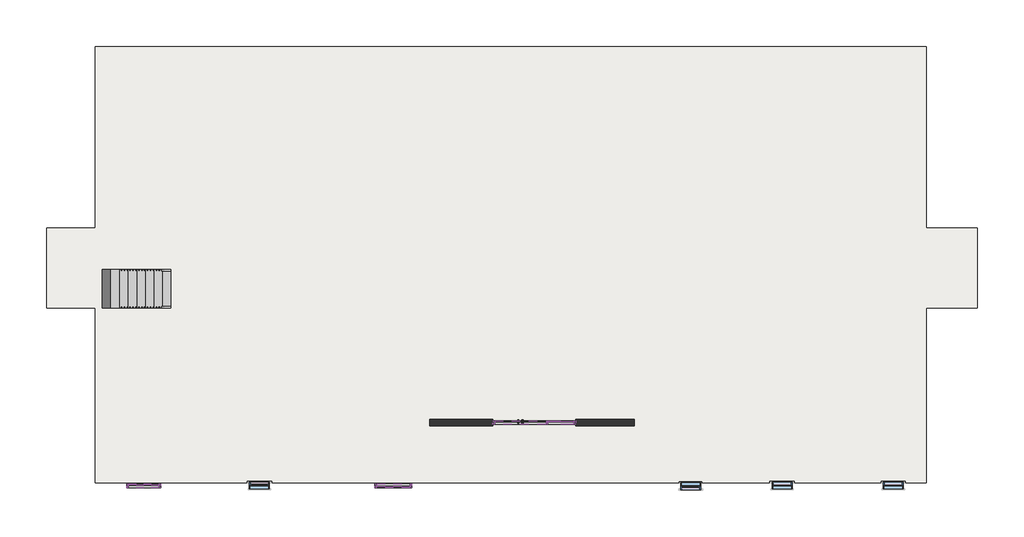
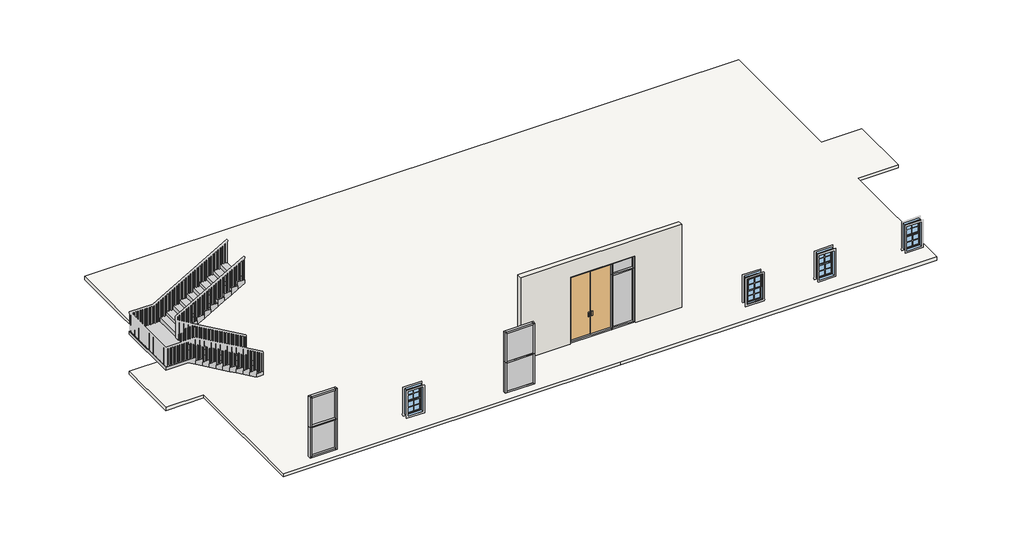
# One storey, part 1 of 3: 25 members, 6 plates, 4 windows, 1 door, 1 slab, 1 stair flight, 1 wall.
"""IFC4 building model written with IfcOpenShell, lengths in millimetres."""

from ifc_helpers import new_model, si_unit, frame, origin, place, context, project, spatial, polyline, outline, extrude, faceted_brep, transform, mapped, element, save
from components import m_door_curtain_wall_double_glass_m_door_curtain_wall_double_f99ce068, rectangular_mullion_65_x_125mm_rectangular_b7ff14d5, rectangular_mullion_65_x_125mm_rectangular_013ac084, rectangular_mullion_65_x_125mm_rectangular_ca84e85e, rectangular_mullion_65_x_125mm_rectangular_f4cebacc, rectangular_mullion_65_x_125mm_rectangular_d33d7bb0, rectangular_mullion_65_x_125mm_rectangular_fcec82ed, rectangular_mullion_65_x_125mm_rectangular_cb623ca7, rectangular_mullion_65_x_125mm_rectangular_e22a5c8f, rectangular_mullion_65_x_125mm_rectangular_b6b0b808, rectangular_mullion_65_x_125mm_rectangular_89386302, rectangular_mullion_65_x_125mm_rectangular_1b222a86, rectangular_mullion_65_x_125mm_rectangular_018360c9, system_panel_glazed_abc17199, system_panel_glazed_3f3a89de, system_panel_glazed_39fbb70d, system_panel_glazed_1607d5b8, m_window_double_hung_700_x_1200mm_9cb858e8

model = new_model("IFC4")

# Units and contexts
model_context = context("Model", 3, world=origin())
ifc_project = project(units=[si_unit("LENGTHUNIT", "METRE", prefix="MILLI")], contexts=[model_context])

# Site, building, storey
site = spatial("IfcSite", under=ifc_project)
building = spatial("IfcBuilding", under=site)
storey = spatial("IfcBuildingStorey", under=building, Elevation=600.0)

# Door
placement = place(None, origin())
m_door_curtain_wall_double_glass_m_door_curtain_wall_double_shape = m_door_curtain_wall_double_glass_m_door_curtain_wall_double_f99ce068(model_context)
element("IfcDoor", 1, ObjectType="M_Door-Curtain-Wall-Double-Glass : M_Door-Curtain-Wall-Double-Glass", at=placement, inside=storey, context=model_context, shape_type="MappedRepresentation", body=[
    mapped(m_door_curtain_wall_double_glass_m_door_curtain_wall_double_shape, transform((5384.8330368, -10653.0592374, 665.0), x_axis=(1.0, 0.0, 0.0), y_axis=(0.0, 1.0, 0.0), z_axis=(0.0, 0.0, 1.0))),
])

# Members
rectangular_mullion_65_x_125mm_rectangular_shape = rectangular_mullion_65_x_125mm_rectangular_b7ff14d5(model_context)
element("IfcMember", 2, ObjectType="Rectangular Mullion : 65 x 125mm rectangular", at=placement, inside=storey, context=model_context, shape_type="MappedRepresentation", body=[
    mapped(rectangular_mullion_65_x_125mm_rectangular_shape, transform((-7258.9169632, -12865.5592374, 3900.0), x_axis=(0.0, 0.0, 1.0), y_axis=(0.0, -1.0, 0.0), z_axis=(1.0, 0.0, 0.0))),
])
element("IfcMember", 3, ObjectType="Rectangular Mullion : 65 x 125mm rectangular", at=placement, inside=storey, context=model_context, shape_type="MappedRepresentation", body=[
    mapped(rectangular_mullion_65_x_125mm_rectangular_shape, transform((-8328.9169632, -12865.5592374, 1050.0), x_axis=(0.0, 0.0, -1.0), y_axis=(0.0, -1.0, 0.0), z_axis=(-1.0, 0.0, 0.0))),
])
rectangular_mullion_65_x_125mm_rectangular_2_shape = rectangular_mullion_65_x_125mm_rectangular_013ac084(model_context)
element("IfcMember", 4, ObjectType="Rectangular Mullion : 65 x 125mm rectangular", at=placement, inside=storey, context=model_context, shape_type="MappedRepresentation", body=[
    mapped(rectangular_mullion_65_x_125mm_rectangular_2_shape, transform((358.5830368, -12865.5592374, 3900.0), x_axis=(0.0, 0.0, 1.0), y_axis=(0.0, 1.0, 0.0), z_axis=(-1.0, 0.0, 0.0))),
])
element("IfcMember", 5, ObjectType="Rectangular Mullion : 65 x 125mm rectangular", at=placement, inside=storey, context=model_context, shape_type="MappedRepresentation", body=[
    mapped(rectangular_mullion_65_x_125mm_rectangular_2_shape, transform((1528.5830368, -12865.5592374, 1050.0), x_axis=(0.0, 0.0, -1.0), y_axis=(0.0, 1.0, 0.0), z_axis=(1.0, 0.0, 0.0))),
])
rectangular_mullion_65_x_125mm_rectangular_3_shape = rectangular_mullion_65_x_125mm_rectangular_ca84e85e(model_context)
element("IfcMember", 6, ObjectType="Rectangular Mullion : 65 x 125mm rectangular", at=placement, inside=storey, context=model_context, shape_type="MappedRepresentation", body=[
    mapped(rectangular_mullion_65_x_125mm_rectangular_3_shape, transform((-7258.9169632, -12865.5592374, 2475.0), x_axis=(0.0, 0.0, 1.0), y_axis=(0.0, -1.0, 0.0), z_axis=(1.0, 0.0, 0.0))),
])
rectangular_mullion_65_x_125mm_rectangular_4_shape = rectangular_mullion_65_x_125mm_rectangular_f4cebacc(model_context)
element("IfcMember", 7, ObjectType="Rectangular Mullion : 65 x 125mm rectangular", at=placement, inside=storey, context=model_context, shape_type="MappedRepresentation", body=[
    mapped(rectangular_mullion_65_x_125mm_rectangular_4_shape, transform((-7193.9169632, -12865.5592374, 1050.0), x_axis=(1.0, 0.0, 0.0), y_axis=(0.0, -1.0, 0.0), z_axis=(0.0, 0.0, -1.0))),
])
element("IfcMember", 8, ObjectType="Rectangular Mullion : 65 x 125mm rectangular", at=placement, inside=storey, context=model_context, shape_type="MappedRepresentation", body=[
    mapped(rectangular_mullion_65_x_125mm_rectangular_4_shape, transform((293.5830368, -12865.5592374, 1050.0), x_axis=(-1.0, 0.0, 0.0), y_axis=(0.0, 1.0, 0.0), z_axis=(0.0, 0.0, -1.0))),
])
element("IfcMember", 9, ObjectType="Rectangular Mullion : 65 x 125mm rectangular", at=placement, inside=storey, context=model_context, shape_type="MappedRepresentation", body=[
    mapped(rectangular_mullion_65_x_125mm_rectangular_4_shape, transform((-8393.9169632, -12865.5592374, 3900.0), x_axis=(-1.0, 0.0, 0.0), y_axis=(0.0, -1.0, 0.0), z_axis=(0.0, 0.0, 1.0))),
])
element("IfcMember", 10, ObjectType="Rectangular Mullion : 65 x 125mm rectangular", at=placement, inside=storey, context=model_context, shape_type="MappedRepresentation", body=[
    mapped(rectangular_mullion_65_x_125mm_rectangular_4_shape, transform((1593.5830368, -12865.5592374, 3900.0), x_axis=(1.0, 0.0, 0.0), y_axis=(0.0, 1.0, 0.0), z_axis=(0.0, 0.0, 1.0))),
])
element("IfcMember", 11, ObjectType="Rectangular Mullion : 65 x 125mm rectangular", at=placement, inside=storey, context=model_context, shape_type="MappedRepresentation", body=[
    mapped(rectangular_mullion_65_x_125mm_rectangular_4_shape, transform((293.5830368, -12865.5592374, 2475.0), x_axis=(-1.0, 0.0, 0.0), y_axis=(0.0, 1.0, 0.0), z_axis=(0.0, 0.0, -1.0))),
])
element("IfcMember", 12, ObjectType="Rectangular Mullion : 65 x 125mm rectangular", at=placement, inside=storey, context=model_context, shape_type="MappedRepresentation", body=[
    mapped(rectangular_mullion_65_x_125mm_rectangular_4_shape, transform((-7193.9169632, -12865.5592374, 2475.0), x_axis=(1.0, 0.0, 0.0), y_axis=(0.0, -1.0, 0.0), z_axis=(0.0, 0.0, -1.0))),
])
element("IfcMember", 13, ObjectType="Rectangular Mullion : 65 x 125mm rectangular", at=placement, inside=storey, context=model_context, shape_type="MappedRepresentation", body=[
    mapped(rectangular_mullion_65_x_125mm_rectangular_4_shape, transform((1593.5830368, -12865.5592374, 2475.0), x_axis=(1.0, 0.0, 0.0), y_axis=(0.0, 1.0, 0.0), z_axis=(0.0, 0.0, 1.0))),
])
element("IfcMember", 14, ObjectType="Rectangular Mullion : 65 x 125mm rectangular", at=placement, inside=storey, context=model_context, shape_type="MappedRepresentation", body=[
    mapped(rectangular_mullion_65_x_125mm_rectangular_4_shape, transform((-8393.9169632, -12865.5592374, 2475.0), x_axis=(-1.0, 0.0, 0.0), y_axis=(0.0, -1.0, 0.0), z_axis=(0.0, 0.0, 1.0))),
])
rectangular_mullion_65_x_125mm_rectangular_5_shape = rectangular_mullion_65_x_125mm_rectangular_d33d7bb0(model_context)
element("IfcMember", 15, ObjectType="Rectangular Mullion : 65 x 125mm rectangular", at=placement, inside=storey, context=model_context, shape_type="MappedRepresentation", body=[
    mapped(rectangular_mullion_65_x_125mm_rectangular_5_shape, transform((358.5830368, -12865.5592374, 2475.0), x_axis=(0.0, 0.0, 1.0), y_axis=(0.0, 1.0, 0.0), z_axis=(-1.0, 0.0, 0.0))),
])
rectangular_mullion_65_x_125mm_rectangular_6_shape = rectangular_mullion_65_x_125mm_rectangular_fcec82ed(model_context)
element("IfcMember", 16, ObjectType="Rectangular Mullion : 65 x 125mm rectangular", at=placement, inside=storey, context=model_context, shape_type="MappedRepresentation", body=[
    mapped(rectangular_mullion_65_x_125mm_rectangular_6_shape, transform((7253.5830368, -10653.0592374, 3750.0), x_axis=(0.0, 0.0, 1.0), y_axis=(0.0, -1.0, 0.0), z_axis=(1.0, 0.0, 0.0))),
])
rectangular_mullion_65_x_125mm_rectangular_7_shape = rectangular_mullion_65_x_125mm_rectangular_cb623ca7(model_context)
element("IfcMember", 17, ObjectType="Rectangular Mullion : 65 x 125mm rectangular", at=placement, inside=storey, context=model_context, shape_type="MappedRepresentation", body=[
    mapped(rectangular_mullion_65_x_125mm_rectangular_7_shape, transform((4483.5830368, -10653.0592374, 600.0), x_axis=(0.0, 0.0, -1.0), y_axis=(0.0, -1.0, 0.0), z_axis=(-1.0, 0.0, 0.0))),
])
element("IfcMember", 18, ObjectType="Rectangular Mullion : 65 x 125mm rectangular", at=placement, inside=storey, context=model_context, shape_type="MappedRepresentation", body=[
    mapped(rectangular_mullion_65_x_125mm_rectangular_7_shape, transform((6286.0830368, -10653.0592374, 3750.0), x_axis=(0.0, 0.0, 1.0), y_axis=(0.0, -1.0, 0.0), z_axis=(1.0, 0.0, 0.0))),
])
element("IfcMember", 19, ObjectType="Rectangular Mullion : 65 x 125mm rectangular", at=placement, inside=storey, context=model_context, shape_type="MappedRepresentation", body=[
    mapped(rectangular_mullion_65_x_125mm_rectangular_6_shape, transform((6351.0830368, -10653.0592374, 600.0), x_axis=(0.0, 0.0, -1.0), y_axis=(0.0, -1.0, 0.0), z_axis=(-1.0, 0.0, 0.0))),
])
rectangular_mullion_65_x_125mm_rectangular_8_shape = rectangular_mullion_65_x_125mm_rectangular_e22a5c8f(model_context)
element("IfcMember", 20, ObjectType="Rectangular Mullion : 65 x 125mm rectangular", at=placement, inside=storey, context=model_context, shape_type="MappedRepresentation", body=[
    mapped(rectangular_mullion_65_x_125mm_rectangular_8_shape, transform((4418.5830368, -10653.0592374, 3750.0), x_axis=(-1.0, 0.0, 0.0), y_axis=(0.0, -1.0, 0.0), z_axis=(0.0, 0.0, 1.0))),
])
rectangular_mullion_65_x_125mm_rectangular_9_shape = rectangular_mullion_65_x_125mm_rectangular_b6b0b808(model_context)
element("IfcMember", 21, ObjectType="Rectangular Mullion : 65 x 125mm rectangular", at=placement, inside=storey, context=model_context, shape_type="MappedRepresentation", body=[
    mapped(rectangular_mullion_65_x_125mm_rectangular_9_shape, transform((4418.5830368, -10653.0592374, 3150.0), x_axis=(-1.0, 0.0, 0.0), y_axis=(0.0, -1.0, 0.0), z_axis=(0.0, 0.0, 1.0))),
])
rectangular_mullion_65_x_125mm_rectangular_10_shape = rectangular_mullion_65_x_125mm_rectangular_89386302(model_context)
element("IfcMember", 22, ObjectType="Rectangular Mullion : 65 x 125mm rectangular", at=placement, inside=storey, context=model_context, shape_type="MappedRepresentation", body=[
    mapped(rectangular_mullion_65_x_125mm_rectangular_10_shape, transform((6318.5830368, -10653.0592374, 600.0), x_axis=(1.0, 0.0, 0.0), y_axis=(0.0, -1.0, 0.0), z_axis=(0.0, 0.0, -1.0))),
])
rectangular_mullion_65_x_125mm_rectangular_11_shape = rectangular_mullion_65_x_125mm_rectangular_1b222a86(model_context)
element("IfcMember", 23, ObjectType="Rectangular Mullion : 65 x 125mm rectangular", at=placement, inside=storey, context=model_context, shape_type="MappedRepresentation", body=[
    mapped(rectangular_mullion_65_x_125mm_rectangular_11_shape, transform((6318.5830368, -10653.0592374, 3150.0), x_axis=(1.0, 0.0, 0.0), y_axis=(0.0, -1.0, 0.0), z_axis=(0.0, 0.0, -1.0))),
])
rectangular_mullion_65_x_125mm_rectangular_12_shape = rectangular_mullion_65_x_125mm_rectangular_018360c9(model_context)
element("IfcMember", 24, ObjectType="Rectangular Mullion : 65 x 125mm rectangular", at=placement, inside=storey, context=model_context, shape_type="MappedRepresentation", body=[
    mapped(rectangular_mullion_65_x_125mm_rectangular_12_shape, transform((7253.5830368, -10653.0592374, 3150.0), x_axis=(0.0, 0.0, 1.0), y_axis=(0.0, -1.0, 0.0), z_axis=(1.0, 0.0, 0.0))),
])
element("IfcMember", 25, ObjectType="Rectangular Mullion : 65 x 125mm rectangular", at=placement, inside=storey, context=model_context, shape_type="MappedRepresentation", body=[
    mapped(rectangular_mullion_65_x_125mm_rectangular_9_shape, transform((7318.5830368, -10653.0592374, 600.0), x_axis=(1.0, 0.0, 0.0), y_axis=(0.0, -1.0, 0.0), z_axis=(0.0, 0.0, -1.0))),
])
element("IfcMember", 26, ObjectType="Rectangular Mullion : 65 x 125mm rectangular", at=placement, inside=storey, context=model_context, shape_type="MappedRepresentation", body=[
    mapped(rectangular_mullion_65_x_125mm_rectangular_8_shape, transform((7318.5830368, -10653.0592374, 3150.0), x_axis=(1.0, 0.0, 0.0), y_axis=(0.0, -1.0, 0.0), z_axis=(0.0, 0.0, -1.0))),
])

# Plates
system_panel_glazed_shape = system_panel_glazed_abc17199(model_context)
element("IfcPlate", 27, ObjectType="System Panel : Glazed", at=placement, inside=storey, context=model_context, shape_type="MappedRepresentation", body=[
    mapped(system_panel_glazed_shape, transform((-7793.9169632, -12865.5592374, 1115.0), x_axis=(1.0, 0.0, 0.0), y_axis=(0.0, 1.0, 0.0), z_axis=(0.0, 0.0, 1.0))),
])
element("IfcPlate", 28, ObjectType="System Panel : Glazed", at=placement, inside=storey, context=model_context, shape_type="MappedRepresentation", body=[
    mapped(system_panel_glazed_shape, transform((-7793.9169632, -12865.5592374, 2507.5), x_axis=(1.0, 0.0, 0.0), y_axis=(0.0, 1.0, 0.0), z_axis=(0.0, 0.0, 1.0))),
])
system_panel_glazed_2_shape = system_panel_glazed_3f3a89de(model_context)
element("IfcPlate", 29, ObjectType="System Panel : Glazed", at=placement, inside=storey, context=model_context, shape_type="MappedRepresentation", body=[
    mapped(system_panel_glazed_2_shape, transform((943.5830368, -12865.5592374, 1115.0), x_axis=(-1.0, 0.0, 0.0), y_axis=(0.0, -1.0, 0.0), z_axis=(0.0, 0.0, 1.0))),
])
element("IfcPlate", 30, ObjectType="System Panel : Glazed", at=placement, inside=storey, context=model_context, shape_type="MappedRepresentation", body=[
    mapped(system_panel_glazed_2_shape, transform((943.5830368, -12865.5592374, 2507.5), x_axis=(-1.0, 0.0, 0.0), y_axis=(0.0, -1.0, 0.0), z_axis=(0.0, 0.0, 1.0))),
])
system_panel_glazed_3_shape = system_panel_glazed_39fbb70d(model_context)
element("IfcPlate", 31, ObjectType="System Panel : Glazed", at=placement, inside=storey, context=model_context, shape_type="MappedRepresentation", body=[
    mapped(system_panel_glazed_3_shape, transform((6802.3330368, -10653.0592374, 665.0), x_axis=(1.0, 0.0, 0.0), y_axis=(0.0, 1.0, 0.0), z_axis=(0.0, 0.0, 1.0))),
])
system_panel_glazed_4_shape = system_panel_glazed_1607d5b8(model_context)
element("IfcPlate", 32, ObjectType="System Panel : Glazed", at=placement, inside=storey, context=model_context, shape_type="MappedRepresentation", body=[
    mapped(system_panel_glazed_4_shape, transform((6802.3330368, -10653.0592374, 3182.5), x_axis=(1.0, 0.0, 0.0), y_axis=(0.0, 1.0, 0.0), z_axis=(0.0, 0.0, 1.0))),
])

# Slab
element("IfcSlab", 33, ObjectType="01-150 floor", at=placement, inside=storey, context=model_context, shape_type="SweptSolid", body=[
    extrude(outline(polyline([(-9493.9169632, 2521.9407626), (19581.0830368, 2521.9407626), (19581.0830368, -3840.5592374), (21381.0830368, -3840.5592374), (21381.0830368, -6640.5592374), (19581.0830368, -6640.5592374), (19581.0830368, -12753.0592374), (5529.3260748, -12753.0592374), (-9493.9169632, -12753.0592374), (-9493.9169632, -6640.5592374), (-11193.9169632, -6640.5592374), (-11193.9169632, -3840.5592374), (-9493.9169632, -3840.5592374), (-9493.9169632, 2521.9407626)])), frame((0.0, 0.0, 450.0), z_axis=(0.0, 0.0, 1.0), x_axis=(1.0, 0.0, 0.0)), (0.0, 0.0, 1.0), 150.0),
])

# Stair flight
element("IfcStairFlight", 34, ObjectType="M_Monolithic Run", at=placement, inside=storey, context=model_context, shape_type="Brep", body=[
    faceted_brep([(-7143.9169632, -6640.5592374, 771.4285714), (-6843.9169632, -6640.5592374, 771.4285714), (-6843.9169632, -5290.5592374, 771.4285714), (-7143.9169632, -5290.5592374, 771.4285714), (-7143.9169632, -6640.5592374, 600.0), (-6843.9169632, -6640.5592374, 600.0), (-6843.9169632, -5290.5592374, 600.0), (-7143.9169632, -5290.5592374, 600.0), (-7443.9169632, -6640.5592374, 942.8571429), (-7143.9169632, -6640.5592374, 942.8571429), (-7143.9169632, -5290.5592374, 942.8571429), (-7443.9169632, -5290.5592374, 942.8571429), (-7443.9169632, -6640.5592374, 770.0944768), (-7146.2516288, -6640.5592374, 600.0), (-7146.2516288, -5290.5592374, 600.0), (-7443.9169632, -5290.5592374, 770.0944768), (-7743.9169632, -6640.5592374, 1114.2857143), (-7443.9169632, -6640.5592374, 1114.2857143), (-7443.9169632, -5290.5592374, 1114.2857143), (-7743.9169632, -5290.5592374, 1114.2857143), (-7743.9169632, -6640.5592374, 941.5230483), (-7743.9169632, -5290.5592374, 941.5230483), (-8043.9169632, -6640.5592374, 1285.7142857), (-7743.9169632, -6640.5592374, 1285.7142857), (-7743.9169632, -5290.5592374, 1285.7142857), (-8043.9169632, -5290.5592374, 1285.7142857), (-8043.9169632, -6640.5592374, 1112.9516197), (-8043.9169632, -5290.5592374, 1112.9516197), (-8343.9169632, -6640.5592374, 1457.1428571), (-8043.9169632, -6640.5592374, 1457.1428571), (-8043.9169632, -5290.5592374, 1457.1428571), (-8343.9169632, -5290.5592374, 1457.1428571), (-8343.9169632, -6640.5592374, 1284.3801911), (-8343.9169632, -5290.5592374, 1284.3801911), (-8643.9169632, -6640.5592374, 1628.5714286), (-8343.9169632, -6640.5592374, 1628.5714286), (-8343.9169632, -5290.5592374, 1628.5714286), (-8643.9169632, -5290.5592374, 1628.5714286), (-8643.9169632, -6640.5592374, 1455.8087625), (-8643.9169632, -5290.5592374, 1455.8087625), (-8943.9169632, -6640.5592374, 1800.0), (-8643.9169632, -6640.5592374, 1800.0), (-8643.9169632, -5290.5592374, 1800.0), (-8943.9169632, -5290.5592374, 1800.0), (-8943.9169632, -6640.5592374, 1627.237334), (-8943.9169632, -5290.5592374, 1627.237334), (-9243.9169632, -6640.5592374, 1971.4285714), (-8943.9169632, -6640.5592374, 1971.4285714), (-8943.9169632, -5290.5592374, 1971.4285714), (-9243.9169632, -5290.5592374, 1971.4285714), (-9243.9169632, -6640.5592374, 1798.6659054), (-9243.9169632, -5290.5592374, 1798.6659054), (-9543.9169632, -6640.5592374, 2142.8571429), (-9243.9169632, -6640.5592374, 2142.8571429), (-9243.9169632, -5290.5592374, 2142.8571429), (-9543.9169632, -5290.5592374, 2142.8571429), (-9543.9169632, -6640.5592374, 1970.0944768), (-9543.9169632, -5290.5592374, 1970.0944768), (-9843.9169632, -6640.5592374, 2314.2857143), (-9543.9169632, -6640.5592374, 2314.2857143), (-9543.9169632, -5290.5592374, 2314.2857143), (-9843.9169632, -5290.5592374, 2314.2857143), (-9843.9169632, -6640.5592374, 2141.5230483), (-10183.7516288, -5290.5592374, 2335.7142857), (-9843.9169632, -5290.5592374, 2335.7142857), (-9843.9169632, -3840.5592374, 2485.7142857), (-11193.9169632, -3840.5592374, 2485.7142857), (-11193.9169632, -6640.5592374, 2485.7142857), (-10183.7516288, -6640.5592374, 2485.7142857), (-9843.9169632, -6640.5592374, 2485.7142857), (-9843.9169632, -5290.5592374, 2485.7142857), (-9843.9169632, -5190.5592374, 2485.7142857), (-9843.9169632, -3840.5592374, 2335.7142857), (-11193.9169632, -3840.5592374, 2335.7142857), (-11193.9169632, -6640.5592374, 2335.7142857), (-10183.7516288, -6640.5592374, 2335.7142857), (-9843.9169632, -5190.5592374, 2335.7142857), (-9843.9169632, -3840.5592374, 2657.1428571), (-9843.9169632, -5190.5592374, 2657.1428571), (-9804.0822977, -5190.5592374, 2657.1428571), (-9543.9169632, -5190.5592374, 2657.1428571), (-9543.9169632, -3840.5592374, 2657.1428571), (-9804.0822977, -3840.5592374, 2657.1428571), (-9543.9169632, -3840.5592374, 2484.3801911), (-9804.0822977, -3840.5592374, 2335.7142857), (-9804.0822977, -5190.5592374, 2335.7142857), (-9543.9169632, -5190.5592374, 2484.3801911), (-9243.9169632, -3840.5592374, 2828.5714286), (-9543.9169632, -3840.5592374, 2828.5714286), (-9543.9169632, -5190.5592374, 2828.5714286), (-9243.9169632, -5190.5592374, 2828.5714286), (-9243.9169632, -3840.5592374, 2655.8087625), (-9243.9169632, -5190.5592374, 2655.8087625), (-8943.9169632, -3840.5592374, 3000.0), (-9243.9169632, -3840.5592374, 3000.0), (-9243.9169632, -5190.5592374, 3000.0), (-8943.9169632, -5190.5592374, 3000.0), (-8943.9169632, -3840.5592374, 2827.237334), (-8943.9169632, -5190.5592374, 2827.237334), (-8643.9169632, -3840.5592374, 3171.4285714), (-8943.9169632, -3840.5592374, 3171.4285714), (-8943.9169632, -5190.5592374, 3171.4285714), (-8643.9169632, -5190.5592374, 3171.4285714), (-8643.9169632, -3840.5592374, 2998.6659054), (-8643.9169632, -5190.5592374, 2998.6659054), (-8343.9169632, -3840.5592374, 3342.8571429), (-8643.9169632, -3840.5592374, 3342.8571429), (-8643.9169632, -5190.5592374, 3342.8571429), (-8343.9169632, -5190.5592374, 3342.8571429), (-8343.9169632, -3840.5592374, 3170.0944768), (-8343.9169632, -5190.5592374, 3170.0944768), (-8043.9169632, -3840.5592374, 3514.2857143), (-8343.9169632, -3840.5592374, 3514.2857143), (-8343.9169632, -5190.5592374, 3514.2857143), (-8043.9169632, -5190.5592374, 3514.2857143), (-8043.9169632, -3840.5592374, 3341.5230483), (-8043.9169632, -5190.5592374, 3341.5230483), (-7743.9169632, -3840.5592374, 3685.7142857), (-8043.9169632, -3840.5592374, 3685.7142857), (-8043.9169632, -5190.5592374, 3685.7142857), (-7743.9169632, -5190.5592374, 3685.7142857), (-7743.9169632, -3840.5592374, 3512.9516197), (-7743.9169632, -5190.5592374, 3512.9516197), (-7443.9169632, -3840.5592374, 3857.1428571), (-7743.9169632, -3840.5592374, 3857.1428571), (-7743.9169632, -5190.5592374, 3857.1428571), (-7443.9169632, -5190.5592374, 3857.1428571), (-7443.9169632, -3840.5592374, 3684.3801911), (-7443.9169632, -5190.5592374, 3684.3801911), (-7143.9169632, -3840.5592374, 4028.5714286), (-7443.9169632, -3840.5592374, 4028.5714286), (-7443.9169632, -5190.5592374, 4028.5714286), (-7143.9169632, -5190.5592374, 4028.5714286), (-7143.9169632, -3840.5592374, 3855.8087625), (-7143.9169632, -5190.5592374, 3855.8087625), (-6843.9169632, -3840.5592374, 4200.0), (-7143.9169632, -3840.5592374, 4200.0), (-7143.9169632, -5190.5592374, 4200.0), (-6843.9169632, -5190.5592374, 4200.0), (-6843.9169632, -3840.5592374, 4027.237334), (-6843.9169632, -5190.5592374, 4027.237334)], [[[0, 1, 2, 3]], [[1, 0, 4, 5]], [[2, 1, 5, 6]], [[3, 2, 6, 7]], [[8, 9, 10, 11]], [[4, 0, 9, 8, 12, 13]], [[0, 3, 10, 9]], [[3, 7, 14, 15, 11, 10]], [[16, 17, 18, 19]], [[17, 16, 20, 12, 8]], [[8, 11, 18, 17]], [[19, 18, 11, 15, 21]], [[22, 23, 24, 25]], [[23, 22, 26, 20, 16]], [[16, 19, 24, 23]], [[25, 24, 19, 21, 27]], [[28, 29, 30, 31]], [[29, 28, 32, 26, 22]], [[22, 25, 30, 29]], [[31, 30, 25, 27, 33]], [[34, 35, 36, 37]], [[35, 34, 38, 32, 28]], [[28, 31, 36, 35]], [[37, 36, 31, 33, 39]], [[40, 41, 42, 43]], [[41, 40, 44, 38, 34]], [[34, 37, 42, 41]], [[43, 42, 37, 39, 45]], [[46, 47, 48, 49]], [[47, 46, 50, 44, 40]], [[40, 43, 48, 47]], [[49, 48, 43, 45, 51]], [[52, 53, 54, 55]], [[53, 52, 56, 50, 46]], [[46, 49, 54, 53]], [[55, 54, 49, 51, 57]], [[58, 59, 60, 61]], [[59, 58, 62, 56, 52]], [[52, 55, 60, 59]], [[61, 60, 55, 57, 63, 64]], [[65, 66, 67, 68, 69, 70, 71]], [[66, 65, 72, 73]], [[67, 66, 73, 74]], [[58, 69, 68, 67, 74, 75, 62]], [[58, 61, 64, 70, 69]], [[71, 70, 64, 76]], [[77, 78, 79, 80, 81, 82]], [[65, 77, 82, 81, 83, 84, 72]], [[65, 71, 78, 77]], [[78, 71, 76, 85, 86, 80, 79]], [[87, 88, 89, 90]], [[88, 87, 91, 83, 81]], [[81, 80, 89, 88]], [[90, 89, 80, 86, 92]], [[93, 94, 95, 96]], [[94, 93, 97, 91, 87]], [[87, 90, 95, 94]], [[96, 95, 90, 92, 98]], [[99, 100, 101, 102]], [[100, 99, 103, 97, 93]], [[93, 96, 101, 100]], [[102, 101, 96, 98, 104]], [[105, 106, 107, 108]], [[106, 105, 109, 103, 99]], [[99, 102, 107, 106]], [[108, 107, 102, 104, 110]], [[111, 112, 113, 114]], [[112, 111, 115, 109, 105]], [[105, 108, 113, 112]], [[114, 113, 108, 110, 116]], [[117, 118, 119, 120]], [[118, 117, 121, 115, 111]], [[111, 114, 119, 118]], [[120, 119, 114, 116, 122]], [[123, 124, 125, 126]], [[124, 123, 127, 121, 117]], [[117, 120, 125, 124]], [[126, 125, 120, 122, 128]], [[129, 130, 131, 132]], [[130, 129, 133, 127, 123]], [[123, 126, 131, 130]], [[132, 131, 126, 128, 134]], [[135, 136, 137, 138]], [[136, 135, 139, 133, 129]], [[129, 132, 137, 136]], [[138, 137, 132, 134, 140]], [[135, 138, 140, 139]], [[5, 4, 13, 14, 7, 6]], [[75, 63, 57, 51, 45, 39, 33, 27, 21, 15, 14, 13, 12, 20, 26, 32, 38, 44, 50, 56, 62]], [[63, 75, 74, 73, 72, 84, 85, 76, 64]], [[85, 84, 83, 91, 97, 103, 109, 115, 121, 127, 133, 139, 140, 134, 128, 122, 116, 110, 104, 98, 92, 86]]]),
])

# Wall
element("IfcWall", 35, ObjectType="01-225 WALL", at=placement, inside=storey, context=model_context, shape_type="SweptSolid", body=[
    extrude(outline(polyline([(4500.0, 9368.5830368), (4500.0, 2218.5830368), (600.0, 2218.5830368), (600.0, 4418.5830368), (3750.0, 4418.5830368), (3750.0, 7318.5830368), (600.0, 7318.5830368), (600.0, 9368.5830368), (4500.0, 9368.5830368)])), frame((0.0, -10765.5592374, 0.0), z_axis=(0.0, 1.0, 0.0), x_axis=(0.0, 0.0, 1.0)), (0.0, 0.0, 1.0), 225.0),
])

# Windows
m_window_double_hung_700_x_1200mm_shape = m_window_double_hung_700_x_1200mm_9cb858e8(model_context)
element("IfcWindow", 36, ObjectType="M_Window-Double-Hung : 700 x 1200mm", at=placement, inside=storey, context=model_context, shape_type="MappedRepresentation", body=[
    mapped(m_window_double_hung_700_x_1200mm_shape, transform((11343.5830368, -12865.5592374, 600.0), x_axis=(-1.0, 0.0, 0.0), y_axis=(0.0, -1.0, 0.0), z_axis=(0.0, 0.0, 1.0))),
])
element("IfcWindow", 37, ObjectType="M_Window-Double-Hung : 700 x 1200mm", at=placement, inside=storey, context=model_context, shape_type="MappedRepresentation", body=[
    mapped(m_window_double_hung_700_x_1200mm_shape, transform((14543.5830368, -12865.5592374, 600.0), x_axis=(1.0, 0.0, 0.0), y_axis=(0.0, 1.0, 0.0), z_axis=(0.0, 0.0, 1.0))),
])
element("IfcWindow", 38, ObjectType="M_Window-Double-Hung : 700 x 1200mm", at=placement, inside=storey, context=model_context, shape_type="MappedRepresentation", body=[
    mapped(m_window_double_hung_700_x_1200mm_shape, transform((18431.0830368, -12865.5592374, 600.0), x_axis=(1.0, 0.0, 0.0), y_axis=(0.0, 1.0, 0.0), z_axis=(0.0, 0.0, 1.0))),
])
element("IfcWindow", 39, ObjectType="M_Window-Double-Hung : 700 x 1200mm", at=placement, inside=storey, context=model_context, shape_type="MappedRepresentation", body=[
    mapped(m_window_double_hung_700_x_1200mm_shape, transform((-3743.9169632, -12865.5592374, 600.0), x_axis=(1.0, 0.0, 0.0), y_axis=(0.0, 1.0, 0.0), z_axis=(0.0, 0.0, 1.0))),
])

save(model, "model.ifc")

# Revit data of these elements
# Type "M_Door-Curtain-Wall-Double-Glass : M_Door-Curtain-Wall-Double-Glass"
#   Type Mark = "53"
#   Assembly Code = "B2030100"
#   Analytic Construction = "<None>"
#   Width [instance default] = 1800 mm
#   Thermal Resistance (R) = 1.7611 (m²·K)/W
#   Swing Angle [instance default] = 90.00°
#   Panel Width [instance default] = 900 mm
#   Offset = 50.8 mm
#   Heat Transfer Coefficient (U) = 0.567826 W/(m²·K)
#   Define Thermal Properties by = 1
#   Function = 1
#   Door Handle Material = Aluminum
#   Glazing = Glass
#   Visual Light Transmittance = 0
#   Solar Heat Gain Coefficient = 0
#   Construction Type Id = ""
# Type "Rectangular Mullion : 65 x 125mm rectangular"
#   built-in parameter 1007304 = 0.410105 (stored number, unit not read)
#   built-in parameter 1007301 = 0.106627 (stored number, unit not read)
#   built-in parameter 1007300 = 0.106627 (stored number, unit not read)
# Type "System Panel : Glazed"
#   Construction Type Id = "GSP4R"
#   Analytic Construction = "1/8 in Pilkington single glazing"
#   Visual Light Transmittance = 0.9
#   Solar Heat Gain Coefficient = 0.86
#   Heat Transfer Coefficient (U) = 6.7069 W/(m²·K)
#   Define Thermal Properties by = 1
# Type "01-150 floor"
#   Description = "Generic Floor (Material By Category), 12\" thick"
#   Assembly Code = "B1010"
#   Type Mark = "G01"
#   Function = 0
#   Layers, outside or top first: 150 mm no material (function 1)
# Type "01-225 WALL"
#   Description = "Generic Wall (Material By Category), 200mm thick"
#   Assembly Code = "B2010"
#   Type Mark = "G06"
#   Layers, outside or top first: 225 mm "01-WHITE WALL" (function 1)
# Type "M_Window-Double-Hung : 700 x 1200mm"
#   Type Mark = "30"
#   Fire Rating = "0.5h"
#   Construction Type Id = "DG-DR"
#   Assembly Code = "B2020100"
#   Analytic Construction = "Double glazing - domestic"
#   Wall Thickness [instance default] = 150 mm
#   Window Inset [instance default] = 0 mm
#   Visual Light Transmittance = 0.81
#   Thermal Resistance (R) = 0.319569 (m²·K)/W
#   Solar Heat Gain Coefficient = 0.76
#   Muntin Width = 547.6 mm
#   Muntin Height = 501.575 mm
#   Interior Wall Closure [instance default] = 35.7 mm
#   Rough Width = 715 mm
#   Rough Height = 1215 mm
#   Frame Extension [instance default] = 31.75 mm
#   Exterior Wall Closure [instance default] = 12.7 mm
#   Extension Jamb [instance default] = 35.7 mm
#   Heat Transfer Coefficient (U) = 3.12929 W/(m²·K)
#   Height = 1200 mm
#   Width = 700 mm
#   Top Muntin Visibility = yes
#   Indicator Visibility [instance default] = yes
#   Extension Jamb Visibility [instance default] = yes
#   Interior Trim Visibility [instance default] = yes
#   Exterior Trim Visibility [instance default] = yes
#   Define Thermal Properties by = 1
#   Bottom Muntin Visibility = yes
#   Muntin Pattern = M_Muntin Pattern_2x2 : M_Muntin Pattern_2x2
#   Interior Trim Material = Wood - Stained
#   Interior Trim = M_Trim-Window-Interior-Flat : Picture Frame
#   Exterior Trim Material = Clad - White
#   Exterior Trim = M_Trim-Window-Exterior-Flat : with Sill
#   Glass Panel Material = Glass
#   Exterior Frame Material = Clad - White
#   Interior Frame Material = Wood - Stained
#   Wall Closure = (empty or 0)
# Element 1 (IfcDoor, "M_Door-Curtain-Wall-Double-Glass : M_Door-Curtain-Wall-Double-Glass")
#   Swing Angle = 90.00°
#   Phase Created = New Construction
#   Materials on its faces: "Aluminum", "Glass"
# Elements 2, 3, 4, 5, 6, 7, 8, 9, 10, 11, 12, 13, 14, 15, 16, 17, 18, 19, 20, 21, 22, 23, 24, 25, 26 (IfcMember, "Rectangular Mullion : 65 x 125mm rectangular")
#   Phase Created = New Construction
#   Materials on its faces: "Aluminum"
# Elements 27, 28, 29, 30, 31, 32 (IfcPlate, "System Panel : Glazed")
#   Phase Created = New Construction
#   Materials on its faces: "Glass"
# Element 33 (IfcSlab, "01-150 floor")
#   built-in parameter 1001955 = 1.5708 (stored number, unit not read)
#   Height Offset From Level = 0 mm
#   Phase Created = New Construction
#   Materials on its faces: "Default Floor"
# Element 34 (IfcStairFlight, "M_Monolithic Run")
#   Phase Created = New Construction
# Element 35 (IfcWall, "01-225 WALL")
#   Top Offset = 0 mm
#   Base Offset = 0 mm
#   wall height = 3900 mm
#   Phase Created = New Construction
#   Base Constraint = 02-DPC
#   Top Constraint = 05-ROOF LEVEL
#   Materials on its faces: "01-WHITE WALL"
# Element 36 (IfcWindow, "M_Window-Double-Hung : 700 x 1200mm")
#   Mark = "100"
#   Window Inset = 0 mm
#   Interior Wall Closure = 35.7 mm
#   Frame Extension = 31.75 mm
#   Exterior Wall Closure = 12.7 mm
#   Interior Trim Visibility = yes
#   Indicator Visibility = yes
#   Exterior Trim Visibility = yes
#   Phase Created = New Construction
#   Materials on its faces: "Wood - Stained", "Glass", "Clad - White"
# Element 37 (IfcWindow, "M_Window-Double-Hung : 700 x 1200mm")
#   Mark = "101"
#   Window Inset = 0 mm
#   Interior Wall Closure = 35.7 mm
#   Frame Extension = 31.75 mm
#   Exterior Wall Closure = 12.7 mm
#   Interior Trim Visibility = yes
#   Indicator Visibility = yes
#   Exterior Trim Visibility = yes
#   Phase Created = New Construction
#   Materials on its faces: "Wood - Stained", "Glass", "Clad - White"
# Element 38 (IfcWindow, "M_Window-Double-Hung : 700 x 1200mm")
#   Mark = "102"
#   Window Inset = 0 mm
#   Interior Wall Closure = 35.7 mm
#   Frame Extension = 31.75 mm
#   Exterior Wall Closure = 12.7 mm
#   Interior Trim Visibility = yes
#   Indicator Visibility = yes
#   Exterior Trim Visibility = yes
#   Phase Created = New Construction
#   Materials on its faces: "Wood - Stained", "Glass", "Clad - White"
# Element 39 (IfcWindow, "M_Window-Double-Hung : 700 x 1200mm")
#   Mark = "103"
#   Window Inset = 0 mm
#   Interior Wall Closure = 35.7 mm
#   Frame Extension = 31.75 mm
#   Exterior Wall Closure = 12.7 mm
#   Interior Trim Visibility = yes
#   Indicator Visibility = yes
#   Exterior Trim Visibility = yes
#   Phase Created = New Construction
#   Materials on its faces: "Wood - Stained", "Glass", "Clad - White"
# Materials
#   "Aluminum": class "Metal", colour RGB 244 245 246, transparency 0, Description = "Aluminum 6061", Cost = 0
#   "Glass": class "Glass", colour RGB 245 245 243, transparency 1, Description = "Soda Lime Glass", Cost = 0
#   "01-WHITE WALL": class "Generic", colour RGB 244 244 244, transparency 0, Description = "Acoustic Ceiling Tile 24 x 48", Cost = 0
#   "Wood - Stained": class "Wood", colour RGB 173 132 96, transparency 0, Cost = 0
#   "Clad - White": class "Wood", colour RGB 245 245 243, transparency 0, Cost = 0
#   "Default Floor": colour RGB 128 128 128, transparency 0, Cost = 0
